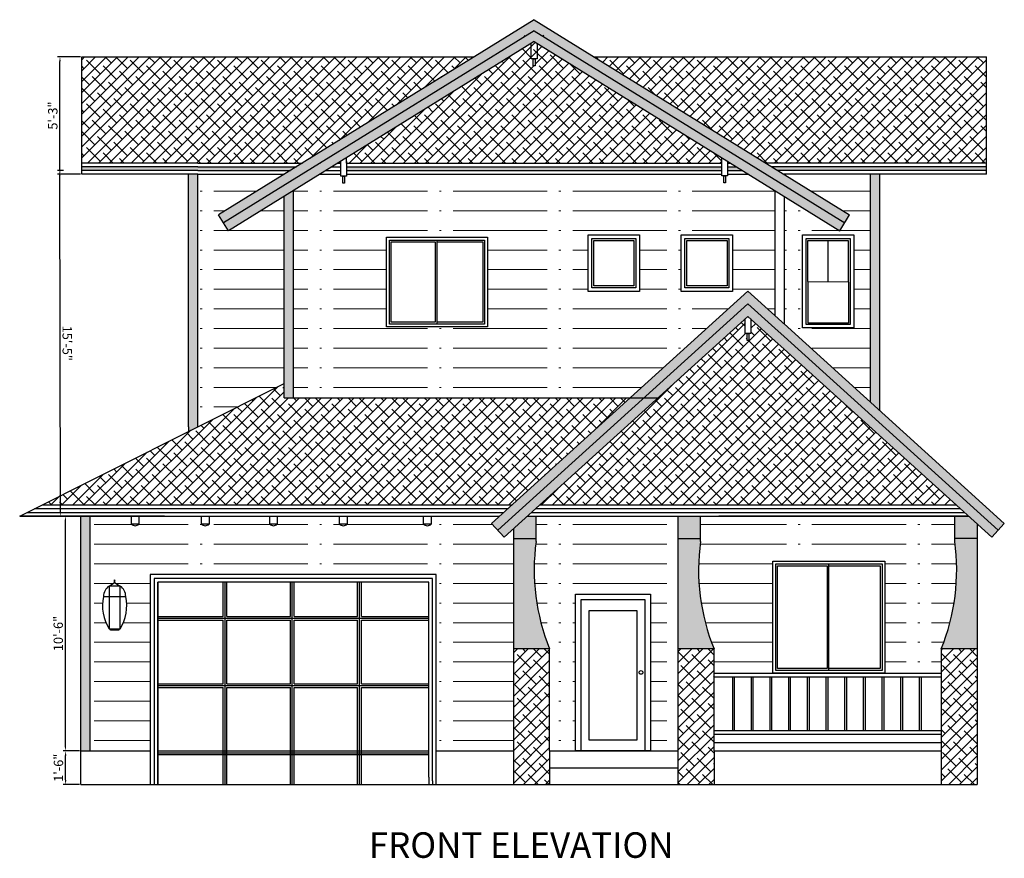
# Model space of a CAD drawing. Units: inches. Extents: x 1838 to 3464, y 573 to 2547.
# Tile 6 of 6: x 2458 to 2985, y 1953 to 2402. Entities that reach past the tile are written whole.
import ezdxf

# ---------------------------------------------------------------- set-up
doc = ezdxf.new("R2010")
doc.units = ezdxf.units.IN
for name, color, linetype, lineweight in [('A-ANNO-DIMS', 2, 'Continuous', 18), ('A-ANNO-TEXT', 7, 'Continuous', 18), ('A-DOOR', 4, 'Continuous', 25), ('A-ELEV', 7, 'Continuous', 25), ('A-ELEV-PATT', 252, 'Continuous', 13), ('A-GLAZ', 3, 'Continuous', 25)]:
    doc.layers.add(name, color=color, linetype=linetype, lineweight=lineweight)
doc.styles.get("Standard").update_dxf_attribs({"font": 'arial.ttf'})
doc.dimstyles.new('ISO-25', dxfattribs={"dimtxt": 5, "dimasz": 2.5, "dimexe": 1.25, "dimexo": 0.625, "dimtad": 1, "dimdec": 0, "dimlunit": 4, "dimtxsty": 'Standard', "dimcen": 2.5, "dimadec": 0, "dimazin": 0, "dimtfac": 1, "dimtdec": 0, "dimtmove": 0, "dimatfit": 3, "dimfxl": 1, "dimarcsym": 0})

# ---------------------------------------------------------------- blocks, each defined once
blk = doc.blocks.new('*U55')
blk.add_lwpolyline([(3.12, 0.01), (0.12, 0.01), (0.12, 84.01), (40.12, 84.01), (40.12, 0.01), (37.12, 0.01)])
for points in [[(37.12, 80.99), (37.12, 0.01), (3.12, 0.01), (3.12, 80.99)], [(33.12, 6.01), (33.12, 74.99), (7.12, 74.99), (7.12, 6.01)]]:
    blk.add_lwpolyline(points, close=True)
blk.add_circle((35.12, 42.01), 1)
blk = doc.blocks.new('*U56')
for p, q in [((1.5, 1.5), (1.5, 58.5)), ((1.5, 58.5), (30, 58.5)), ((30, 1.5), (30, 58.5)), ((30, 58.5), (58.5, 58.5)), ((58.5, 58.5), (58.5, 1.5)), ((30, 1.5), (1.5, 1.5)), ((58.5, 1.5), (30, 1.5))]:
    blk.add_line(p, q)
blk.add_lwpolyline([(0, 0), (0, 60), (60, 60), (60, 0)], close=True)
for points in [[(29, 57.5), (29, 2.5), (2.5, 2.5), (2.5, 57.5), (29, 57.5)], [(30, 57.5), (57.5, 57.5), (57.5, 2.5), (30, 2.5)]]:
    blk.add_lwpolyline(points)
blk = doc.blocks.new('*U57')
for p, q in [((1.5, 1.5), (1.5, 46.5)), ((1.5, 46.5), (27, 46.5)), ((27, 1.5), (27, 46.5)), ((27, 46.5), (52.5, 46.5)), ((52.5, 46.5), (52.5, 1.5)), ((27, 1.5), (1.5, 1.5)), ((52.5, 1.5), (27, 1.5))]:
    blk.add_line(p, q)
blk.add_lwpolyline([(0, 0), (0, 48), (54, 48), (54, 0)], close=True)
for points in [[(26, 45.5), (26, 2.5), (2.5, 2.5), (2.5, 45.5), (26, 45.5)], [(27, 45.5), (51.5, 45.5), (51.5, 2.5), (27, 2.5)]]:
    blk.add_lwpolyline(points)
blk = doc.blocks.new('*D58')
at = {"layer": 'A-ANNO-DIMS', "color": 0, "lineweight": -2, "transparency": 16777216}
for p, q in [((2490.16, 2010.36), (2481.42, 2010.36)), ((2482.67, 1994.86), (2482.67, 2007.86)), ((2490.16, 1992.36), (2481.42, 1992.36))]:
    blk.add_line(p, q, dxfattribs=at)
at = {"layer": 'A-ANNO-DIMS', "color": 0, "lineweight": 100, "transparency": 16777216}
for points in [[(2482.25, 2007.86), (2483.08, 2007.86), (2482.67, 2010.36)], [(2482.25, 1994.86), (2483.08, 1994.86), (2482.67, 1992.36)]]:
    blk.add_solid(points, dxfattribs=at)
at = {"layer": 'Defpoints', "color": 0, "lineweight": 100, "transparency": 16777216}
for p in [(2482.67, 2010.36), (2490.78, 2010.36), (2490.78, 1992.36)]:
    blk.add_point(p, dxfattribs=at)
at = {"layer": 'A-ANNO-DIMS', "color": 0, "transparency": 16777216, "insert": (2479.49, 2001.36), "char_height": 5, "attachment_point": 5, "rotation": 90}
blk.add_mtext('1\'-6"', dxfattribs=at)
blk = doc.blocks.new('*D59')
at = {"layer": 'A-ANNO-DIMS', "color": 0, "lineweight": -2, "transparency": 16777216}
for p, q in [((2490.16, 2136.08), (2481.31, 2136.08)), ((2482.56, 2012.86), (2482.56, 2133.58)), ((2490.16, 2010.36), (2481.31, 2010.36))]:
    blk.add_line(p, q, dxfattribs=at)
at = {"layer": 'A-ANNO-DIMS', "color": 0, "lineweight": 100, "transparency": 16777216}
for points in [[(2482.15, 2133.58), (2482.98, 2133.58), (2482.56, 2136.08)], [(2482.15, 2012.86), (2482.98, 2012.86), (2482.56, 2010.36)]]:
    blk.add_solid(points, dxfattribs=at)
at = {"layer": 'Defpoints', "color": 0, "lineweight": 100, "transparency": 16777216}
for p in [(2482.56, 2136.08), (2490.78, 2136.08), (2490.78, 2010.36)]:
    blk.add_point(p, dxfattribs=at)
at = {"layer": 'A-ANNO-DIMS', "color": 0, "transparency": 16777216, "insert": (2479.38, 2073.22), "char_height": 5, "attachment_point": 5, "rotation": 90}
blk.add_mtext('10\'-6"', dxfattribs=at)
blk = doc.blocks.new('*D60')
at = {"layer": 'A-ANNO-DIMS', "color": 0, "lineweight": -2, "transparency": 16777216}
for p, q in [((2481.57, 2321.07), (2478.26, 2321.07)), ((2479.88, 2138.57), (2479.52, 2318.57)), ((2481.94, 2136.08), (2478.63, 2136.07))]:
    blk.add_line(p, q, dxfattribs=at)
at = {"layer": 'A-ANNO-DIMS', "color": 0, "lineweight": 100, "transparency": 16777216}
for points in [[(2479.94, 2318.57), (2479.1, 2318.57), (2479.51, 2321.07)], [(2480.29, 2138.57), (2479.46, 2138.57), (2479.88, 2136.07)]]:
    blk.add_solid(points, dxfattribs=at)
at = {"layer": 'Defpoints', "color": 0, "lineweight": 100, "transparency": 16777216}
for p in [(2479.51, 2321.07), (2482.2, 2321.08), (2482.56, 2136.08)]:
    blk.add_point(p, dxfattribs=at)
at = {"layer": 'A-ANNO-DIMS', "color": 0, "transparency": 16777216, "insert": (2482.88, 2228.58), "char_height": 5, "attachment_point": 5, "rotation": 270.1132}
blk.add_mtext('15\'-5"', dxfattribs=at)
blk = doc.blocks.new('*D61')
at = {"layer": 'A-ANNO-DIMS', "color": 0, "lineweight": -2, "transparency": 16777216}
for p, q in [((2490.65, 2381.95), (2478.39, 2381.95)), ((2479.64, 2321.58), (2479.64, 2379.45)), ((2490.65, 2319.08), (2478.39, 2319.08))]:
    blk.add_line(p, q, dxfattribs=at)
at = {"layer": 'A-ANNO-DIMS', "color": 0, "lineweight": 100, "transparency": 16777216}
for points in [[(2479.22, 2379.45), (2480.06, 2379.45), (2479.64, 2381.95)], [(2479.22, 2321.58), (2480.06, 2321.58), (2479.64, 2319.08)]]:
    blk.add_solid(points, dxfattribs=at)
at = {"layer": 'Defpoints', "color": 0, "lineweight": 100, "transparency": 16777216}
for p in [(2479.64, 2381.95), (2491.28, 2381.95), (2491.28, 2319.08)]:
    blk.add_point(p, dxfattribs=at)
at = {"layer": 'A-ANNO-DIMS', "color": 0, "transparency": 16777216, "insert": (2476.46, 2350.51), "char_height": 5, "attachment_point": 5, "rotation": 90}
blk.add_mtext('5\'-3"', dxfattribs=at)

msp = doc.modelspace()

# ---------------------------------------------------------------- hatches: boundary and pattern name
at = {"layer": 'A-ELEV-PATT'}
h = msp.add_hatch(color=256, dxfattribs=at)
h.dxf.hatch_style = 1
h.paths.add_polyline_path([(2734.55, 2122.5), (2734.55, 2124.14), (2722.48, 2124.14), (2722.48, 2064.94), (2741.81, 2064.94, -0.131307)])
h.paths.add_polyline_path([(2822.59, 2122.5), (2822.59, 2124.14), (2810.52, 2124.14), (2810.52, 2064.94), (2829.85, 2064.94, -0.131307)])
h.paths.add_polyline_path([(2822.59, 2136.08), (2810.52, 2136.08), (2810.52, 2124.14), (2822.59, 2124.14)])
h.paths.add_polyline_path([(2734.55, 2136.08), (2729.93, 2136.08), (2722.48, 2129.33), (2722.48, 2124.14), (2734.55, 2124.14)])
h.paths.add_polyline_path([(2970.78, 2124.14), (2958.71, 2124.14), (2958.71, 2122.5, -0.131307), (2951.45, 2064.94), (2970.78, 2064.94)])
h.paths.add_polyline_path([(2970.78, 2131.79), (2966.05, 2136.08), (2958.71, 2136.08), (2958.71, 2124.14), (2970.78, 2124.14)])
h.paths.add_polyline_path([(2792.31, 2199.32), (2784.86, 2199.32), (2710.74, 2132.19), (2714.1, 2128.48)])
h.paths.add_polyline_path([(2799.75, 2199.32), (2792.31, 2199.32), (2714.1, 2128.48), (2717.45, 2124.78)])
h.paths.add_polyline_path([(2867.39, 2232.18), (2862.39, 2236.71), (2847.99, 2249.76), (2792.31, 2199.32), (2799.75, 2199.32), (2847.99, 2243.01), (2849.48, 2241.66), (2849.54, 2241.66), (2849.54, 2241.6), (2862.39, 2229.97), (2867.39, 2225.44), (2978.52, 2124.78), (2981.88, 2128.48)])
h.paths.add_polyline_path([(2867.39, 2238.93), (2862.39, 2243.46), (2847.99, 2256.5), (2784.86, 2199.32), (2792.31, 2199.32), (2847.99, 2249.76), (2862.39, 2236.71), (2867.39, 2232.18), (2981.88, 2128.48), (2985.24, 2132.19)])
h.paths.add_polyline_path([(2733.5, 2395.95), (2899.77, 2293.05), (2902.4, 2297.3), (2733.5, 2401.83), (2564.6, 2297.3), (2567.23, 2293.05)])
h.paths.add_polyline_path([(2733.5, 2390.07), (2897.14, 2288.8), (2899.77, 2293.05), (2733.5, 2395.95), (2567.23, 2293.05), (2569.86, 2288.8)])
h.paths.add_polyline_path([(2833.98, 2323.08), (2633.09, 2323.08), (2633.09, 2321.08), (2833.98, 2321.08)], flags=17)
h.paths.add_polyline_path([(2841.76, 2323.08), (2837.03, 2323.08), (2837.03, 2321.08), (2844.99, 2321.08)], flags=17)
h.paths.add_polyline_path([(2606.2, 2323.05), (2599.78, 2323.08), (2553.38, 2323.08), (2491.28, 2323.08), (2491.28, 2321.08), (2553.38, 2321.08), (2599.78, 2321.08), (2603.03, 2321.09)])
h.paths.add_polyline_path([(2975.73, 2323.08), (2913.62, 2323.08), (2867.22, 2323.08), (2860.76, 2323.08), (2863.99, 2321.08), (2867.22, 2321.08), (2913.62, 2321.08), (2975.73, 2321.08)])
h = msp.add_hatch(dxfattribs=at)
h.set_pattern_fill('ANSI38', color=256, scale=1.3)
h.paths.add_polyline_path([(2491.28, 2381.95), (2491.28, 2325.08), (2553.38, 2325.08), (2599.78, 2325.08), (2609.47, 2325.08), (2701.38, 2381.95)])
h.paths.add_polyline_path([(2833.98, 2325.08), (2833.98, 2326.04), (2833.98, 2327.89), (2735.05, 2389.11), (2735.05, 2388.72), (2735.05, 2380.9), (2734.01, 2380.9), (2734.01, 2377.2), (2733.08, 2377.2), (2733.08, 2380.9), (2735.05, 2380.9), (2735.05, 2388.72), (2735.05, 2389.11), (2733.5, 2390.07), (2633.09, 2327.93), (2633.09, 2325.08)])
h.paths.add_polyline_path([(2913.62, 2325.08), (2975.73, 2325.08), (2975.73, 2381.95), (2765.63, 2381.95), (2857.53, 2325.08), (2867.22, 2325.08)])
h.paths.add_polyline_path([(2867.39, 2225.44), (2862.39, 2229.97), (2849.54, 2241.6), (2849.54, 2233.84), (2848.5, 2233.84), (2848.5, 2230.14), (2847.56, 2230.14), (2847.56, 2233.84), (2846.49, 2233.84), (2846.49, 2241.66), (2736.55, 2142.08), (2959.42, 2142.08)])
h.paths.add_polyline_path([(2829.85, 2064.94), (2810.52, 2064.94), (2810.52, 2010.36), (2810.52, 1992.36), (2829.85, 1992.36), (2829.85, 2010.36), (2829.85, 2019.36)])
h.paths.add_polyline_path([(2741.81, 2064.94), (2722.48, 2064.94), (2722.48, 2010.36), (2722.48, 1992.36), (2741.81, 1992.36), (2741.81, 2010.36)])
h.paths.add_polyline_path([(2970.78, 2064.94), (2951.45, 2064.94), (2951.45, 2010.36), (2951.45, 1992.36), (2970.78, 1992.36), (2970.78, 2010.36)])
h.paths.add_polyline_path([(2711.92, 2142.08), (2721.66, 2142.08), (2784.86, 2199.32), (2599.61, 2199.32), (2599.61, 2206.99), (2470.06, 2142.08)])
h = msp.add_hatch(dxfattribs=at)
h.set_pattern_fill('ACAD_ISO04W100', color=256, scale=2.1)
h.paths.add_polyline_path([(2604.61, 2199.32), (2784.86, 2199.32), (2847.99, 2256.5), (2862.39, 2243.46), (2862.39, 2310.3), (2848.22, 2319.08), (2837.03, 2319.08), (2837.03, 2318.23), (2835.99, 2318.23), (2835.99, 2314.53), (2835.05, 2314.53), (2835.05, 2318.23), (2833.98, 2318.23), (2833.98, 2319.08), (2633.09, 2319.08), (2633.09, 2318.01), (2632.05, 2318.01), (2632.05, 2314.31), (2631.11, 2314.31), (2631.11, 2318.01), (2630.04, 2318.01), (2630.04, 2319.08), (2618.78, 2319.08), (2604.61, 2310.3)])
h.paths.add_polyline_path([(2654.51, 2285.34), (2708.51, 2285.34), (2708.51, 2237.34), (2654.51, 2237.34)], flags=16)
h.paths.add_polyline_path([(2656.01, 2283.84), (2681.51, 2283.84), (2707.01, 2283.84), (2707.01, 2238.84), (2681.51, 2238.84), (2656.01, 2238.84)], flags=0)
h.paths.add_polyline_path([(2680.51, 2239.84), (2680.51, 2282.84), (2657.01, 2282.84), (2657.01, 2239.84)], flags=0)
h.paths.add_polyline_path([(2681.51, 2282.84), (2706.01, 2282.84), (2706.01, 2239.84), (2681.51, 2239.84)], flags=0)
h.paths.add_polyline_path([(2762.39, 2286.62), (2789.97, 2286.62), (2789.97, 2256.31), (2762.39, 2256.31)], flags=16)
h.paths.add_polyline_path([(2764.39, 2284.62), (2787.97, 2284.62), (2787.97, 2258.31), (2764.39, 2258.31)], flags=0)
h.paths.add_polyline_path([(2765.39, 2283.62), (2786.97, 2283.62), (2786.97, 2259.31), (2765.39, 2259.31)], flags=0)
h.paths.add_polyline_path([(2812.2, 2286.62), (2839.77, 2286.62), (2839.77, 2256.31), (2812.2, 2256.31)], flags=16)
h.paths.add_polyline_path([(2814.2, 2284.62), (2837.77, 2284.62), (2837.77, 2258.31), (2814.2, 2258.31)], flags=0)
h.paths.add_polyline_path([(2815.2, 2283.62), (2836.77, 2283.62), (2836.77, 2259.31), (2815.2, 2259.31)], flags=0)
h.paths.add_polyline_path([(2722.48, 2129.33), (2717.45, 2124.78), (2710.74, 2132.19), (2715.03, 2136.08), (2711.92, 2136.08), (2678.36, 2136.08), (2678.36, 2131.79, -0.417833), (2674.3, 2131.79), (2674.3, 2136.08), (2633.38, 2136.08), (2633.38, 2131.79, -0.417833), (2629.32, 2131.79), (2629.32, 2136.08), (2595.98, 2136.08), (2595.98, 2131.79, -0.417833), (2591.92, 2131.79), (2591.92, 2136.08), (2559.46, 2136.08), (2559.46, 2131.79, -0.417833), (2555.4, 2131.79), (2555.4, 2136.08), (2521.92, 2136.08), (2521.92, 2131.79, -0.417833), (2517.86, 2131.79), (2517.86, 2136.08), (2495.78, 2136.08), (2495.78, 2118.36), (2495.78, 2010.36), (2528.01, 2010.36), (2528.01, 2104.75), (2681.06, 2104.75), (2681.06, 2010.36), (2722.48, 2010.36)])
h.paths.add_polyline_path([(2511.47, 2075.09), (2506.38, 2075.09, -0.206237), (2502.99, 2093.04, -0.252701), (2506.01, 2098.63), (2508.93, 2100.54, -0.282395), (2508.93, 2101.96, -0.282395), (2508.93, 2100.54), (2511.84, 2098.63, -0.252701), (2514.86, 2093.04, -0.206237)], flags=16)
h.paths.add_polyline_path([(2810.52, 2136.08), (2734.55, 2136.08), (2734.55, 2122.5, 0.131307), (2741.81, 2064.94), (2741.81, 2010.36), (2755.73, 2010.36), (2755.73, 2094.37), (2795.73, 2094.37), (2795.73, 2010.36), (2810.52, 2010.36)])
h.paths.add_polyline_path([(2829.85, 2064.94), (2829.85, 2051.96), (2861.36, 2051.96), (2861.36, 2111.96), (2921.36, 2111.96), (2921.36, 2051.96), (2951.45, 2051.96), (2951.45, 2064.94, 0.131307), (2958.71, 2122.5), (2958.71, 2136.08), (2832.31, 2136.08), (2822.59, 2136.08), (2822.59, 2122.5, 0.131307)])
h = msp.add_hatch(color=256, dxfattribs=at)
h.dxf.hatch_style = 1
h.paths.add_polyline_path([(2553.38, 2319.08), (2548.38, 2319.08), (2548.38, 2183.82), (2548.38, 2181.32), (2553.38, 2183.82)])
h.paths.add_polyline_path([(2918.62, 2319.08), (2913.62, 2319.08), (2913.62, 2197.05), (2918.62, 2192.52)])
h = msp.add_hatch(dxfattribs=at)
h.set_pattern_fill('ACAD_ISO04W100', color=256, scale=2.1)
h.paths.add_polyline_path([(2599.61, 2307.21), (2569.86, 2288.8), (2564.6, 2297.3), (2599.61, 2318.97), (2599.61, 2319.08), (2553.38, 2319.08), (2553.38, 2183.82), (2599.61, 2206.99)])
h.paths.add_polyline_path([(2913.62, 2319.08), (2867.39, 2319.08), (2867.39, 2318.97), (2902.4, 2297.3), (2897.14, 2288.8), (2867.39, 2307.21), (2867.39, 2238.93), (2913.62, 2197.05)])
h.paths.add_polyline_path([(2877.13, 2236.84), (2877.13, 2286.62), (2904.7, 2286.62), (2904.7, 2236.84)], flags=16)
h.paths.add_polyline_path([(2879.13, 2238.6), (2879.13, 2284.62), (2902.7, 2284.62), (2902.7, 2238.6)], flags=0)
h.paths.add_polyline_path([(2880.31, 2239.43), (2880.13, 2283.62), (2901.7, 2283.62), (2901.89, 2239.43)], flags=0)
h = msp.add_hatch(color=256, dxfattribs=at)
h.dxf.hatch_style = 1
h.paths.add_polyline_path([(2495.78, 2118.36), (2495.78, 2136.08), (2490.78, 2136.08), (2490.78, 2118.36), (2490.78, 2010.36), (2495.78, 2010.36)])
h.paths.add_polyline_path([(2604.61, 2310.3), (2599.61, 2307.21), (2599.61, 2199.32), (2604.61, 2199.32)])

# ---------------------------------------------------------------- linework, layer by layer
at = {"layer": 'A-ELEV'}
for p, q in [((2733.5, 2401.83), (2564.6, 2297.3)), ((2733.5, 2401.83), (2902.4, 2297.3)), ((2733.5, 2395.95), (2567.23, 2293.05)), ((2728.24, 2393.33), (2728.75, 2393.01)), ((2733.5, 2395.95), (2899.77, 2293.05)), ((2738.76, 2393.33), (2738.25, 2393.01)), ((2733.5, 2390.07), (2569.86, 2288.8)), ((2732, 2388.72), (2732, 2389.14)), ((2733.5, 2390.07), (2897.14, 2288.8)), ((2735.05, 2388.72), (2735.05, 2389.11)), ((2491.28, 2319.08), (2491.28, 2381.95)), ((2491.28, 2381.95), (2701.38, 2381.95)), ((2765.63, 2381.95), (2975.73, 2381.95)), ((2975.73, 2319.08), (2975.73, 2381.95)), ((2553.38, 2325.08), (2491.28, 2325.08)), ((2553.38, 2325.08), (2599.78, 2325.08)), ((2599.78, 2325.08), (2609.47, 2325.08)), ((2618.78, 2325.08), (2618.98, 2325.08)), ((2628.48, 2325.08), (2630.04, 2325.08)), ((2630.04, 2325.83), (2630.04, 2326.04)), ((2633.09, 2325.08), (2633.09, 2327.93)), ((2633.09, 2325.08), (2833.98, 2325.08)), ((2833.98, 2326.04), (2833.98, 2327.89)), ((2837.03, 2325.08), (2838.52, 2325.08)), ((2848.02, 2325.08), (2848.22, 2325.08)), ((2867.22, 2325.08), (2857.53, 2325.08)), ((2913.62, 2325.08), (2867.22, 2325.08)), ((2975.73, 2325.08), (2913.62, 2325.08)), ((2553.38, 2323.08), (2491.28, 2323.08)), ((2553.38, 2321.08), (2491.28, 2321.08)), ((2553.38, 2323.08), (2599.78, 2323.08)), ((2553.38, 2321.08), (2599.78, 2321.08)), ((2599.78, 2323.08), (2606.2, 2323.05)), ((2599.78, 2321.08), (2603.03, 2321.09)), ((2622.01, 2321.08), (2630.04, 2321.08)), ((2625.25, 2323.08), (2630.04, 2323.08)), ((2633.09, 2323.08), (2833.98, 2323.08)), ((2633.09, 2321.08), (2833.98, 2321.08)), ((2837.03, 2323.08), (2841.76, 2323.08)), ((2837.03, 2321.08), (2844.99, 2321.08)), ((2867.22, 2323.08), (2860.76, 2323.08)), ((2867.22, 2321.08), (2863.99, 2321.08)), ((2913.62, 2323.08), (2867.22, 2323.08)), ((2913.62, 2321.08), (2867.22, 2321.08)), ((2975.73, 2323.08), (2913.62, 2323.08)), ((2975.73, 2321.08), (2913.62, 2321.08)), ((2553.38, 2319.08), (2491.28, 2319.08)), ((2553.38, 2319.08), (2491.28, 2319.08)), ((2548.38, 2183.82), (2548.38, 2319.08)), ((2553.38, 2183.82), (2553.38, 2319.08)), ((2553.38, 2319.08), (2599.78, 2319.08)), ((2599.61, 2319.08), (2599.78, 2319.08)), ((2599.61, 2318.97), (2599.61, 2319.08)), ((2618.78, 2319.08), (2630.04, 2319.08)), ((2633.09, 2319.08), (2833.98, 2319.08)), ((2837.03, 2319.08), (2848.22, 2319.08)), ((2913.62, 2319.08), (2867.22, 2319.08)), ((2867.22, 2319.08), (2867.39, 2319.08)), ((2867.39, 2319.08), (2867.39, 2318.97)), ((2913.62, 2197.05), (2913.62, 2319.08)), ((2975.73, 2319.08), (2913.62, 2319.08)), ((2918.62, 2192.52), (2918.62, 2319.08)), ((2604.61, 2199.32), (2604.61, 2310.3)), ((2862.39, 2310.3), (2862.39, 2243.46)), ((2599.61, 2199.32), (2599.61, 2307.21)), ((2867.39, 2307.21), (2867.39, 2238.93)), ((2569.86, 2288.8), (2564.6, 2297.3)), ((2897.14, 2288.8), (2902.4, 2297.3)), ((2847.99, 2256.5), (2710.74, 2132.19)), ((2847.99, 2256.5), (2862.39, 2243.46)), ((2847.99, 2249.76), (2714.1, 2128.48)), ((2847.99, 2249.76), (2862.39, 2236.71)), ((2847.99, 2243.01), (2717.45, 2124.78)), ((2847.99, 2243.01), (2862.39, 2229.97)), ((2862.39, 2243.46), (2868.13, 2238.26)), ((2862.39, 2236.71), (2867.39, 2232.18)), ((2867.39, 2238.93), (2985.24, 2132.19)), ((2862.39, 2229.97), (2867.39, 2225.44)), ((2867.39, 2232.18), (2981.88, 2128.48)), ((2867.39, 2225.44), (2978.52, 2124.78)), ((2458.08, 2136.08), (2599.61, 2206.99)), ((2599.61, 2199.32), (2799.75, 2199.32)), ((2548.38, 2183.82), (2548.38, 2181.32)), ((2470.06, 2142.08), (2711.92, 2142.08)), ((2711.92, 2142.08), (2721.66, 2142.08)), ((2736.55, 2142.08), (2959.42, 2142.08)), ((2535.66, 2136.08), (2458.08, 2136.08)), ((2458.08, 2136.08), (2711.92, 2136.08)), ((2462.08, 2138.08), (2711.92, 2138.08)), ((2466.07, 2140.08), (2711.92, 2140.08)), ((2490.78, 2118.36), (2490.78, 2136.08)), ((2490.78, 2136.08), (2535.66, 2136.08)), ((2495.78, 2118.36), (2495.78, 2136.08)), ((2711.92, 2140.08), (2719.45, 2140.08)), ((2711.92, 2138.08), (2717.24, 2138.08)), ((2711.92, 2136.08), (2715.03, 2136.08)), ((2729.93, 2136.08), (2966.05, 2136.08)), ((2732.14, 2138.08), (2963.84, 2138.08)), ((2734.35, 2140.08), (2961.63, 2140.08)), ((2734.55, 2122.5), (2734.55, 2136.08)), ((2810.52, 2136.08), (2810.52, 2010.36)), ((2822.59, 2122.5), (2822.59, 2136.08)), ((2966.05, 2136.08), (2832.31, 2136.08)), ((2958.71, 2122.5), (2958.71, 2136.08)), ((2717.45, 2124.78), (2710.74, 2132.19)), ((2970.78, 2131.79), (2970.78, 2010.36)), ((2978.52, 2124.78), (2985.24, 2132.19)), ((2722.48, 2129.33), (2722.48, 2010.36)), ((2722.48, 2124.14), (2734.79, 2124.14)), ((2810.52, 2124.14), (2822.83, 2124.14)), ((2970.78, 2124.14), (2958.47, 2124.14)), ((2490.78, 2010.36), (2490.78, 2118.36)), ((2495.78, 2010.36), (2495.78, 2118.36)), ((2506.01, 2098.63), (2508.93, 2100.54)), ((2508.93, 2100.54), (2508.93, 2101.96)), ((2508.93, 2100.54), (2511.84, 2098.63)), ((2532.01, 1992.36), (2532.01, 2100.75)), ((2502.99, 2093.04), (2514.77, 2093.04)), ((2741.81, 2064.94), (2722.48, 2064.94)), ((2741.81, 2010.36), (2741.81, 2064.94)), ((2829.85, 2064.94), (2810.52, 2064.94)), ((2829.85, 2010.36), (2829.85, 2064.94)), ((2970.78, 2064.94), (2951.45, 2064.94)), ((2951.45, 2064.94), (2951.45, 2010.36)), ((2829.85, 2051.96), (2951.45, 2051.96)), ((2829.85, 2049.96), (2951.45, 2049.96)), ((2829.85, 2021.36), (2829.85, 2049.96)), ((2839.85, 2021.36), (2839.85, 2049.96)), ((2840.85, 2021.36), (2840.85, 2049.96)), ((2849.85, 2021.36), (2849.85, 2049.96)), ((2850.85, 2021.36), (2850.85, 2049.96)), ((2859.85, 2021.36), (2859.85, 2049.96)), ((2860.85, 2021.36), (2860.85, 2049.96)), ((2869.85, 2021.36), (2869.85, 2049.96)), ((2870.85, 2021.36), (2870.85, 2049.96)), ((2879.85, 2021.36), (2879.85, 2049.96)), ((2880.85, 2021.36), (2880.85, 2049.96)), ((2889.85, 2021.36), (2889.85, 2049.96)), ((2890.85, 2021.36), (2890.85, 2049.96)), ((2899.85, 2021.36), (2899.85, 2049.96)), ((2900.85, 2021.36), (2900.85, 2049.96)), ((2909.85, 2021.36), (2909.85, 2049.96)), ((2910.85, 2021.36), (2910.85, 2049.96)), ((2919.85, 2021.36), (2919.85, 2049.96)), ((2920.85, 2021.36), (2920.85, 2049.96)), ((2929.85, 2021.36), (2929.85, 2049.96)), ((2930.85, 2021.36), (2930.85, 2049.96)), ((2939.85, 2021.36), (2939.85, 2049.96)), ((2940.85, 2021.36), (2940.85, 2049.96)), ((2829.85, 2021.36), (2951.45, 2021.36)), ((2829.85, 2010.36), (2829.85, 2019.36)), ((2829.85, 2019.36), (2951.45, 2019.36)), ((2829.85, 2014.86), (2951.45, 2014.86)), ((2490.78, 1992.36), (2490.78, 2010.36)), ((2490.78, 2010.36), (2528.01, 2010.36)), ((2532.01, 1992.36), (2532.01, 2010.36)), ((2681.06, 2010.36), (2722.48, 2010.36)), ((2722.48, 2010.36), (2722.48, 1992.36)), ((2741.81, 2010.36), (2741.81, 1992.36)), ((2741.81, 2010.36), (2810.52, 2010.36)), ((2810.52, 2010.36), (2810.52, 1992.36)), ((2829.85, 2010.36), (2829.85, 1992.36)), ((2829.85, 2010.36), (2951.45, 2010.36)), ((2951.45, 2010.36), (2951.45, 1992.36)), ((2970.78, 2010.36), (2970.78, 1992.36)), ((2741.81, 2001.36), (2810.52, 2001.36)), ((2530.01, 1994.36), (2530.01, 1992.36)), ((2532.01, 1996.36), (2532.01, 1992.36)), ((2677.06, 1996.36), (2677.06, 1992.36)), ((2679.06, 1994.36), (2679.06, 1992.36)), ((2490.78, 1992.36), (2970.78, 1992.36))]:
    msp.add_line(p, q, dxfattribs=at)
for points in [[(2735.05, 2388.72), (2735.05, 2380.9), (2732, 2380.9), (2732, 2388.72)], [(2633.09, 2325.83), (2633.09, 2318.01), (2630.04, 2318.01), (2630.04, 2325.83)], [(2837.03, 2326.04), (2837.03, 2318.23), (2833.98, 2318.23), (2833.98, 2326.04)], [(2849.48, 2241.66), (2849.54, 2241.66), (2849.54, 2233.84), (2846.49, 2233.84), (2846.49, 2241.66)]]:
    msp.add_lwpolyline(points, dxfattribs=at)
for points in [[(2733.08, 2380.9), (2734.01, 2380.9), (2734.01, 2377.2), (2733.08, 2377.2)], [(2631.11, 2318.01), (2632.05, 2318.01), (2632.05, 2314.31), (2631.11, 2314.31)], [(2835.05, 2318.23), (2835.99, 2318.23), (2835.99, 2314.53), (2835.05, 2314.53)], [(2847.56, 2233.84), (2848.5, 2233.84), (2848.5, 2230.14), (2847.56, 2230.14)], [(2517.86, 2136.08), (2521.92, 2136.08), (2521.92, 2131.79), (2517.86, 2131.79)], [(2555.4, 2136.08), (2559.46, 2136.08), (2559.46, 2131.79), (2555.4, 2131.79)], [(2591.92, 2136.08), (2595.98, 2136.08), (2595.98, 2131.79), (2591.92, 2131.79)], [(2629.32, 2136.08), (2633.38, 2136.08), (2633.38, 2131.79), (2629.32, 2131.79)], [(2674.3, 2136.08), (2678.36, 2136.08), (2678.36, 2131.79), (2674.3, 2131.79)], [(2506.01, 2075.67), (2511.84, 2075.67), (2511.84, 2098.63), (2506.01, 2098.63)], [(2506.65, 2075.67), (2511.24, 2075.67), (2511.24, 2075.09), (2506.65, 2075.09)]]:
    msp.add_lwpolyline(points, close=True, dxfattribs=at)
for centre, radius, start, end in [((2519.89, 2133.79), 2.85, 224.6464, 315.3536), ((2557.43, 2133.79), 2.85, 224.6464, 315.3536), ((2593.95, 2133.79), 2.85, 224.6464, 315.3536), ((2631.35, 2133.79), 2.85, 224.6464, 315.3536), ((2676.33, 2133.79), 2.85, 224.6464, 315.3536), ((2845.9, 2107.31), 112.38, 172.2281, 202.1503), ((2933.93, 2107.31), 112.38, 172.2281, 202.1503), ((2847.37, 2107.31), 112.38, 337.8497, 7.7719), ((2509.67, 2093.04), 6.68, 123.2729, 180), ((2510.08, 2101.25), 1.36, 148.4611, 211.5389), ((2507.77, 2101.25), 1.36, 328.4611, 31.5389), ((2508.18, 2093.04), 6.68, 0, 56.7271), ((2525.53, 2088), 23.09, 167.3917, 212.2944), ((2492.32, 2088), 23.09, 327.7056, 12.6083)]:
    msp.add_arc(centre, radius, start, end, dxfattribs=at)
at = {"layer": 'A-GLAZ'}
for p, q in [((2890.91, 2261.73), (2890.91, 2283.62)), ((2880.22, 2261.53), (2901.79, 2261.62)), ((2567.01, 2082.36), (2567.01, 2100.75)), ((2568.01, 1992.36), (2568.01, 2100.75)), ((2569.01, 2082.36), (2569.01, 2100.75)), ((2603.01, 2082.36), (2603.01, 2100.75)), ((2604.01, 1992.36), (2604.01, 2100.75)), ((2605.01, 2082.36), (2605.01, 2100.75)), ((2639.01, 2082.36), (2639.01, 2100.75)), ((2640.01, 1992.36), (2640.01, 2100.75)), ((2641.01, 2082.36), (2641.01, 2100.75)), ((2532.01, 2082.36), (2567.01, 2082.36)), ((2569.01, 2082.36), (2603.01, 2082.36)), ((2605.01, 2082.36), (2639.01, 2082.36)), ((2641.01, 2082.36), (2677.06, 2082.36)), ((2532.01, 2081.36), (2677.06, 2081.36)), ((2532.01, 2080.36), (2567.01, 2080.36)), ((2567.01, 2046.36), (2567.01, 2080.36)), ((2569.01, 2080.36), (2603.01, 2080.36)), ((2569.01, 2046.36), (2569.01, 2080.36)), ((2603.01, 2046.36), (2603.01, 2080.36)), ((2605.01, 2080.36), (2639.01, 2080.36)), ((2605.01, 2046.36), (2605.01, 2080.36)), ((2639.01, 2046.36), (2639.01, 2080.36)), ((2641.01, 2080.36), (2677.06, 2080.36)), ((2641.01, 2046.36), (2641.01, 2080.36)), ((2532.01, 2046.36), (2567.01, 2046.36)), ((2532.01, 2045.36), (2677.06, 2045.36)), ((2569.01, 2046.36), (2603.01, 2046.36)), ((2605.01, 2046.36), (2639.01, 2046.36)), ((2641.01, 2046.36), (2677.06, 2046.36)), ((2532.01, 2044.36), (2567.01, 2044.36)), ((2567.01, 1992.36), (2567.01, 2044.36)), ((2569.01, 1992.36), (2569.01, 2044.36)), ((2569.01, 2044.36), (2603.01, 2044.36)), ((2603.01, 1992.36), (2603.01, 2044.36)), ((2605.01, 1992.36), (2605.01, 2044.36)), ((2605.01, 2044.36), (2639.01, 2044.36)), ((2639.01, 1992.36), (2639.01, 2044.36)), ((2641.01, 1992.36), (2641.01, 2044.36)), ((2641.01, 2044.36), (2677.06, 2044.36)), ((2532.01, 2010.36), (2677.06, 2010.36)), ((2532.01, 2009.36), (2677.06, 2009.36)), ((2532.01, 2008.36), (2677.06, 2008.36))]:
    msp.add_line(p, q, dxfattribs=at)
for points in [[(2762.39, 2286.62), (2789.97, 2286.62), (2789.97, 2256.31), (2762.39, 2256.31)], [(2764.39, 2284.62), (2787.97, 2284.62), (2787.97, 2258.31), (2764.39, 2258.31)], [(2765.39, 2283.62), (2786.97, 2283.62), (2786.97, 2259.31), (2765.39, 2259.31)], [(2812.2, 2286.62), (2839.77, 2286.62), (2839.77, 2256.31), (2812.2, 2256.31)], [(2814.2, 2284.62), (2837.77, 2284.62), (2837.77, 2258.31), (2814.2, 2258.31)], [(2815.2, 2283.62), (2836.77, 2283.62), (2836.77, 2259.31), (2815.2, 2259.31)], [(2877.13, 2286.62), (2904.7, 2286.62), (2904.7, 2236.84), (2877.13, 2236.84)], [(2879.13, 2284.62), (2902.7, 2284.62), (2902.7, 2238.6), (2879.13, 2238.6)], [(2880.13, 2283.62), (2901.7, 2283.62), (2901.89, 2239.43), (2880.31, 2239.43)], [(2528.01, 1992.36), (2681.06, 1992.36), (2681.06, 2104.75), (2528.01, 2104.75)]]:
    msp.add_lwpolyline(points, close=True, dxfattribs=at)
for points in [[(2679.06, 1994.36), (2679.06, 2102.75), (2530.01, 2102.75), (2530.01, 1994.36)], [(2677.06, 1996.36), (2677.06, 2100.75), (2532.01, 2100.75), (2532.01, 1996.36)]]:
    msp.add_lwpolyline(points, dxfattribs=at)

# ---------------------------------------------------------------- block references
at = {"layer": 'A-DOOR'}
msp.add_blockref('*U55', (2755.61, 2010.36), dxfattribs=at)
at = {"layer": 'A-GLAZ'}
for name, p in [('*U57', (2654.51, 2237.34)), ('*U56', (2861.36, 2051.96))]:
    msp.add_blockref(name, p, dxfattribs=at)

# ---------------------------------------------------------------- texts
at = {"layer": 'A-ANNO-TEXT', "insert": (2645.06, 1966.8), "char_height": 13.6813, "attachment_point": 1}
msp.add_mtext_dynamic_manual_height_columns('FRONT ELEVATION', width=275.9918, gutter_width=68.41, heights=[0], dxfattribs=at)

# ---------------------------------------------------------------- dimensions: what is measured, and where the dimension line sits
at = {"layer": 'A-ANNO-DIMS'}
for base, p1, p2, picture, middle in [((2479.64, 2381.95), (2491.28, 2319.08), (2491.28, 2381.95), '*D61', (2476.46, 2350.51)), ((2482.56, 2136.08), (2490.78, 2010.36), (2490.78, 2136.08), '*D59', (2479.38, 2073.22)), ((2482.67, 2010.36), (2490.78, 1992.36), (2490.78, 2010.36), '*D58', (2479.49, 2001.36))]:
    dim = msp.add_linear_dim(base=base, p1=p1, p2=p2, angle=90, dimstyle='ISO-25', override={"dimclrd": 0, "dimclre": 0, "dimclrt": 0}, dxfattribs=at)
    dim.commit()
    dim.dimension.update_dxf_attribs({"geometry": picture, "text_midpoint": middle})
dim = msp.add_aligned_dim(p1=(2482.56, 2136.08), p2=(2482.2, 2321.08), distance=2.68, dimstyle='ISO-25', override={"dimclrd": 0, "dimclre": 0, "dimclrt": 0}, dxfattribs=at)
dim.commit()
dim.dimension.update_dxf_attribs({"geometry": '*D60', "text_midpoint": (2482.88, 2228.58)})

doc.saveas('drawing.dxf')
